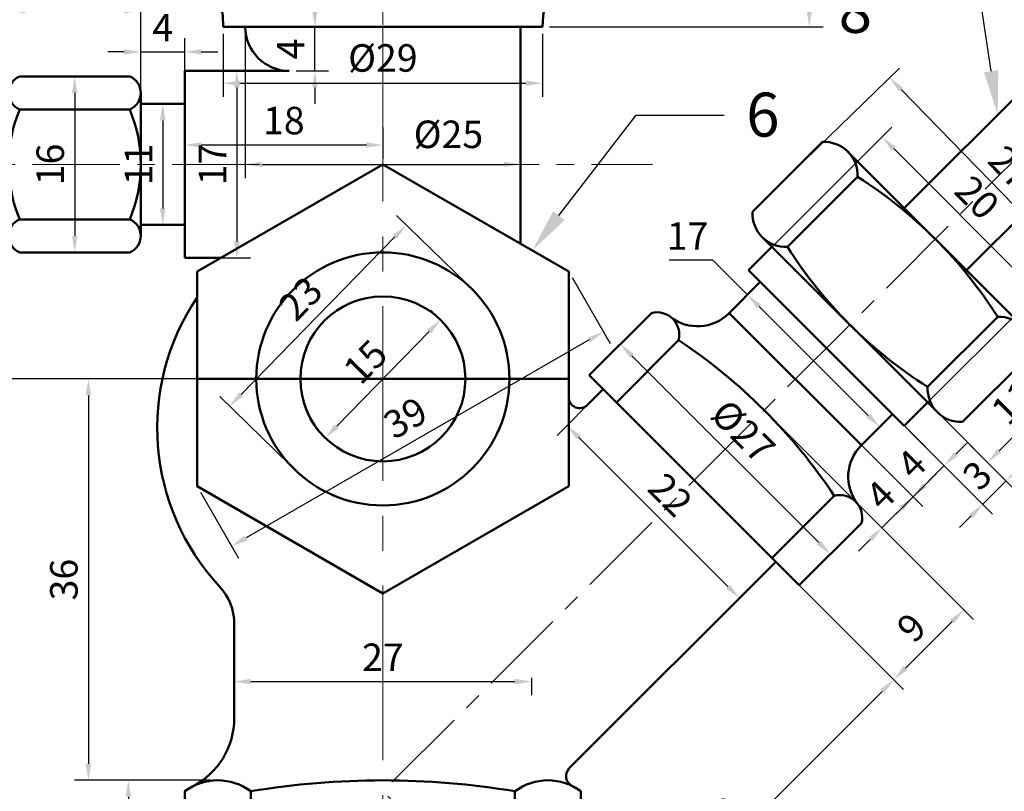
# Model space of a CAD drawing. Units: millimetres. Extents: x -414 to 17, y 81 to 417.
# Tile 3 of 7: x -341 to -252, y 143 to 214. Entities that reach past the tile are written whole.
import ezdxf
from ezdxf import colors
from ezdxf.entities.mleader import LeaderData, LeaderLine
from ezdxf.math import Vec2, Vec3

# ---------------------------------------------------------------- set-up
doc = ezdxf.new("R2010")
doc.units = ezdxf.units.MM
doc.header["$LTSCALE"] = 0.5
doc.linetypes.add('CENTER', pattern=[50.8, 31.75, -6.35, 6.35, -6.35])
for name, color, linetype, lineweight in [('M-CNTR', 1, 'CENTER', 18), ('M-DIMS', 2, 'Continuous', 25), ('M-OUTL', 7, 'Continuous', 50)]:
    doc.layers.add(name, color=color, linetype=linetype, lineweight=lineweight)
doc.styles.get("Standard").update_dxf_attribs({"font": 'arial.ttf'})
doc.dimstyles.new('ISO-25', dxfattribs={"dimtxt": 2.5, "dimasz": 1.5, "dimexe": 1.25, "dimexo": 0.625, "dimtad": 1, "dimtoh": 1, "dimdec": 0, "dimtxsty": 'Standard', "dimcen": 2.5, "dimadec": 0, "dimazin": 0, "dimtfac": 1, "dimtdec": 0, "dimtmove": 0, "dimatfit": 3, "dimfxl": 1, "dimarcsym": 0})

# ---------------------------------------------------------------- blocks, each defined once
blk = doc.blocks.new('*D20')
at = {"layer": 'Defpoints', "color": 0, "ltscale": 0.5, "transparency": 16777216}
for p in [(-281.414, 222.961), (-269.748, 222.961), (-293.993, 212.961)]:
    blk.add_point(p, dxfattribs=at)
at = {"layer": 'M-DIMS', "color": 0, "lineweight": -2, "ltscale": 0.5, "transparency": 16777216}
for p, q in [((-280.789, 222.961), (-268.498, 222.961)), ((-269.748, 214.461), (-269.748, 221.461)), ((-293.368, 212.961), (-268.498, 212.961))]:
    blk.add_line(p, q, dxfattribs=at)
at = {"layer": 'M-DIMS', "color": 0, "ltscale": 0.5, "transparency": 16777216}
for points in [[(-269.998, 221.461), (-269.498, 221.461), (-269.748, 222.961)], [(-269.998, 214.461), (-269.498, 214.461), (-269.748, 212.961)]]:
    blk.add_solid(points, dxfattribs=at)
at = {"layer": 'M-DIMS', "color": 0, "ltscale": 0.5, "transparency": 16777216, "insert": (-271.649, 217.961), "char_height": 2.5, "attachment_point": 5, "rotation": 90}
blk.add_mtext('10', dxfattribs=at)
blk = doc.blocks.new('*D23')
at = {"layer": 'Defpoints', "color": 0, "ltscale": 0.5, "transparency": 16777216}
for p in [(-322.993, 212.961), (-293.993, 212.961), (-293.993, 207.844)]:
    blk.add_point(p, dxfattribs=at)
at = {"layer": 'M-DIMS', "color": 0, "lineweight": -2, "ltscale": 0.5, "transparency": 16777216}
for p, q in [((-322.993, 212.336), (-322.993, 206.594)), ((-293.993, 212.336), (-293.993, 206.594)), ((-321.493, 207.844), (-295.493, 207.844))]:
    blk.add_line(p, q, dxfattribs=at)
at = {"layer": 'M-DIMS', "color": 0, "ltscale": 0.5, "transparency": 16777216}
for points in [[(-321.493, 208.094), (-321.493, 207.594), (-322.993, 207.844)], [(-295.493, 208.094), (-295.493, 207.594), (-293.993, 207.844)]]:
    blk.add_solid(points, dxfattribs=at)
at = {"layer": 'M-DIMS', "color": 0, "ltscale": 0.5, "transparency": 16777216, "insert": (-308.493, 209.815), "char_height": 2.5, "attachment_point": 5}
blk.add_mtext('%%C29', dxfattribs=at)
blk = doc.blocks.new('*D24')
at = {"layer": 'Defpoints', "color": 0, "ltscale": 0.5, "transparency": 16777216}
for p in [(-316.993, 212.961), (-314.671, 212.961), (-316.993, 208.961)]:
    blk.add_point(p, dxfattribs=at)
at = {"layer": 'M-DIMS', "color": 0, "lineweight": -2, "ltscale": 0.5, "transparency": 16777216}
for p, q in [((-314.671, 214.461), (-314.671, 215.961)), ((-316.368, 212.961), (-313.421, 212.961)), ((-314.671, 208.961), (-314.671, 212.961)), ((-316.368, 208.961), (-313.421, 208.961)), ((-314.671, 207.461), (-314.671, 205.961))]:
    blk.add_line(p, q, dxfattribs=at)
at = {"layer": 'M-DIMS', "color": 0, "ltscale": 0.5, "transparency": 16777216}
for points in [[(-314.921, 214.461), (-314.421, 214.461), (-314.671, 212.961)], [(-314.921, 207.461), (-314.421, 207.461), (-314.671, 208.961)]]:
    blk.add_solid(points, dxfattribs=at)
at = {"layer": 'M-DIMS', "color": 0, "ltscale": 0.5, "transparency": 16777216, "insert": (-316.546, 210.961), "char_height": 2.5, "attachment_point": 5, "rotation": 90}
blk.add_mtext('4', dxfattribs=at)
blk = doc.blocks.new('*D25')
at = {"layer": 'Defpoints', "color": 0, "ltscale": 0.5, "transparency": 16777216}
for p in [(-326.493, 204.436), (-308.493, 204.436), (-326.493, 202.223)]:
    blk.add_point(p, dxfattribs=at)
at = {"layer": 'M-DIMS', "color": 0, "lineweight": -2, "ltscale": 0.5, "transparency": 16777216}
for p, q in [((-326.493, 203.811), (-326.493, 200.973)), ((-308.493, 203.811), (-308.493, 200.973)), ((-309.993, 202.223), (-324.993, 202.223))]:
    blk.add_line(p, q, dxfattribs=at)
at = {"layer": 'M-DIMS', "color": 0, "ltscale": 0.5, "transparency": 16777216}
for points in [[(-324.993, 202.473), (-324.993, 201.973), (-326.493, 202.223)], [(-309.993, 202.473), (-309.993, 201.973), (-308.493, 202.223)]]:
    blk.add_solid(points, dxfattribs=at)
at = {"layer": 'M-DIMS', "color": 0, "ltscale": 0.5, "transparency": 16777216, "insert": (-317.493, 204.125), "char_height": 2.5, "attachment_point": 5}
blk.add_mtext('18', dxfattribs=at)
blk = doc.blocks.new('*D26')
at = {"layer": 'Defpoints', "color": 0, "ltscale": 0.5, "transparency": 16777216}
for p in [(-320.993, 212.961), (-295.993, 203.103), (-295.993, 200.461)]:
    blk.add_point(p, dxfattribs=at)
at = {"layer": 'M-DIMS', "color": 0, "lineweight": -2, "ltscale": 0.5, "transparency": 16777216}
for p, q in [((-320.993, 212.336), (-320.993, 199.211)), ((-295.993, 202.478), (-295.993, 199.211)), ((-319.493, 200.461), (-297.493, 200.461))]:
    blk.add_line(p, q, dxfattribs=at)
at = {"layer": 'M-DIMS', "color": 0, "ltscale": 0.5, "transparency": 16777216}
for points in [[(-319.493, 200.711), (-319.493, 200.211), (-320.993, 200.461)], [(-297.493, 200.711), (-297.493, 200.211), (-295.993, 200.461)]]:
    blk.add_solid(points, dxfattribs=at)
at = {"layer": 'M-DIMS', "color": 0, "ltscale": 0.5, "transparency": 16777216, "insert": (-302.537, 202.873), "char_height": 2.5, "attachment_point": 5}
blk.add_mtext('%%C25', dxfattribs=at)
blk = doc.blocks.new('*D27')
at = {"layer": 'Defpoints', "color": 0, "ltscale": 0.5, "transparency": 16777216}
for p in [(-325.219, 208.961), (-325.219, 191.961), (-321.764, 191.961)]:
    blk.add_point(p, dxfattribs=at)
at = {"layer": 'M-DIMS', "color": 0, "lineweight": -2, "ltscale": 0.5, "transparency": 16777216}
for p, q in [((-324.594, 208.961), (-320.514, 208.961)), ((-321.764, 207.461), (-321.764, 193.461)), ((-324.594, 191.961), (-320.514, 191.961))]:
    blk.add_line(p, q, dxfattribs=at)
at = {"layer": 'M-DIMS', "color": 0, "ltscale": 0.5, "transparency": 16777216}
for points in [[(-322.014, 207.461), (-321.514, 207.461), (-321.764, 208.961)], [(-322.014, 193.461), (-321.514, 193.461), (-321.764, 191.961)]]:
    blk.add_solid(points, dxfattribs=at)
at = {"layer": 'M-DIMS', "color": 0, "ltscale": 0.5, "transparency": 16777216, "insert": (-323.644, 200.461), "char_height": 2.5, "attachment_point": 5, "rotation": 90}
blk.add_mtext('17', dxfattribs=at)
blk = doc.blocks.new('*D28')
at = {"layer": 'Defpoints', "color": 0, "ltscale": 0.5, "transparency": 16777216}
for p in [(-328.493, 205.961), (-328.493, 194.961), (-328.493, 194.961)]:
    blk.add_point(p, dxfattribs=at)
at = {"layer": 'M-DIMS', "color": 0, "lineweight": -2, "ltscale": 0.5, "transparency": 16777216}
for p, q in [((-329.118, 205.961), (-329.743, 205.961)), ((-328.493, 204.461), (-328.493, 196.461)), ((-329.118, 194.961), (-329.743, 194.961))]:
    blk.add_line(p, q, dxfattribs=at)
at = {"layer": 'M-DIMS', "color": 0, "ltscale": 0.5, "transparency": 16777216}
for points in [[(-328.743, 204.461), (-328.243, 204.461), (-328.493, 205.961)], [(-328.743, 196.461), (-328.243, 196.461), (-328.493, 194.961)]]:
    blk.add_solid(points, dxfattribs=at)
at = {"layer": 'M-DIMS', "color": 0, "ltscale": 0.5, "transparency": 16777216, "insert": (-330.373, 200.461), "char_height": 2.5, "attachment_point": 5, "rotation": 90}
blk.add_mtext('11', dxfattribs=at)
blk = doc.blocks.new('*D29')
at = {"layer": 'Defpoints', "color": 0, "ltscale": 0.5, "transparency": 16777216}
for p in [(-326.493, 210.694), (-330.493, 205.961), (-326.493, 205.961)]:
    blk.add_point(p, dxfattribs=at)
at = {"layer": 'M-DIMS', "color": 0, "lineweight": -2, "ltscale": 0.5, "transparency": 16777216}
for p, q in [((-330.493, 206.586), (-330.493, 211.944)), ((-326.493, 206.586), (-326.493, 211.944)), ((-331.993, 210.694), (-333.493, 210.694)), ((-330.493, 210.694), (-326.493, 210.694)), ((-324.993, 210.694), (-323.493, 210.694))]:
    blk.add_line(p, q, dxfattribs=at)
at = {"layer": 'M-DIMS', "color": 0, "ltscale": 0.5, "transparency": 16777216}
for points in [[(-331.993, 210.944), (-331.993, 210.444), (-330.493, 210.694)], [(-324.993, 210.944), (-324.993, 210.444), (-326.493, 210.694)]]:
    blk.add_solid(points, dxfattribs=at)
at = {"layer": 'M-DIMS', "color": 0, "ltscale": 0.5, "transparency": 16777216, "insert": (-328.493, 212.569), "char_height": 2.5, "attachment_point": 5}
blk.add_mtext('4', dxfattribs=at)
blk = doc.blocks.new('*D30')
at = {"layer": 'Defpoints', "color": 0, "ltscale": 0.5, "transparency": 16777216}
for p in [(-330.493, 214.444), (-330.493, 209.265), (-342.493, 205.101)]:
    blk.add_point(p, dxfattribs=at)
at = {"layer": 'M-DIMS', "color": 0, "lineweight": -2, "ltscale": 0.5, "transparency": 16777216}
for p, q in [((-342.493, 205.726), (-342.493, 215.694)), ((-330.493, 209.89), (-330.493, 215.694)), ((-340.993, 214.444), (-331.993, 214.444))]:
    blk.add_line(p, q, dxfattribs=at)
at = {"layer": 'M-DIMS', "color": 0, "ltscale": 0.5, "transparency": 16777216}
for points in [[(-340.993, 214.694), (-340.993, 214.194), (-342.493, 214.444)], [(-331.993, 214.694), (-331.993, 214.194), (-330.493, 214.444)]]:
    blk.add_solid(points, dxfattribs=at)
at = {"layer": 'M-DIMS', "color": 0, "ltscale": 0.5, "transparency": 16777216, "insert": (-336.493, 216.324), "char_height": 2.5, "attachment_point": 5}
blk.add_mtext('12', dxfattribs=at)
blk = doc.blocks.new('*D31')
at = {"layer": 'Defpoints', "color": 0, "ltscale": 0.5, "transparency": 16777216}
for p in [(-336.493, 208.461), (-336.493, 192.461), (-336.493, 192.461)]:
    blk.add_point(p, dxfattribs=at)
at = {"layer": 'M-DIMS', "color": 0, "lineweight": -2, "ltscale": 0.5, "transparency": 16777216}
for p, q in [((-337.118, 208.461), (-337.743, 208.461)), ((-336.493, 206.961), (-336.493, 193.961)), ((-337.118, 192.461), (-337.743, 192.461))]:
    blk.add_line(p, q, dxfattribs=at)
at = {"layer": 'M-DIMS', "color": 0, "ltscale": 0.5, "transparency": 16777216}
for points in [[(-336.743, 206.961), (-336.243, 206.961), (-336.493, 208.461)], [(-336.743, 193.961), (-336.243, 193.961), (-336.493, 192.461)]]:
    blk.add_solid(points, dxfattribs=at)
at = {"layer": 'M-DIMS', "color": 0, "ltscale": 0.5, "transparency": 16777216, "insert": (-338.394, 200.461), "char_height": 2.5, "attachment_point": 5, "rotation": 90}
blk.add_mtext('16', dxfattribs=at)
blk = doc.blocks.new('*D37')
at = {"layer": 'Defpoints', "color": 0, "ltscale": 0.5, "transparency": 16777216}
for p in [(-338.493, 222.961), (-374.146, 180.961), (-308.493, 180.961)]:
    blk.add_point(p, dxfattribs=at)
at = {"layer": 'M-DIMS', "color": 0, "lineweight": -2, "ltscale": 0.5, "transparency": 16777216}
for p, q in [((-339.118, 222.961), (-375.396, 222.961)), ((-374.146, 221.461), (-374.146, 182.461)), ((-309.118, 180.961), (-375.396, 180.961))]:
    blk.add_line(p, q, dxfattribs=at)
at = {"layer": 'M-DIMS', "color": 0, "ltscale": 0.5, "transparency": 16777216}
for points in [[(-374.396, 221.461), (-373.896, 221.461), (-374.146, 222.961)], [(-374.396, 182.461), (-373.896, 182.461), (-374.146, 180.961)]]:
    blk.add_solid(points, dxfattribs=at)
at = {"layer": 'M-DIMS', "color": 0, "ltscale": 0.5, "transparency": 16777216, "insert": (-376.027, 201.961), "char_height": 2.5, "attachment_point": 5, "rotation": 90}
blk.add_mtext('42', dxfattribs=at)
blk = doc.blocks.new('*D41')
at = {"layer": 'Defpoints', "color": 0, "ltscale": 0.5, "transparency": 16777216}
for p in [(-383.576, 200.461), (-351.797, 200.461), (-308.493, 115.461)]:
    blk.add_point(p, dxfattribs=at)
at = {"layer": 'M-DIMS', "color": 0, "lineweight": -2, "ltscale": 0.5, "transparency": 16777216}
for p, q in [((-352.422, 200.461), (-384.826, 200.461)), ((-383.576, 116.961), (-383.576, 198.961)), ((-309.118, 115.461), (-384.826, 115.461))]:
    blk.add_line(p, q, dxfattribs=at)
at = {"layer": 'M-DIMS', "color": 0, "ltscale": 0.5, "transparency": 16777216}
for points in [[(-383.826, 198.961), (-383.326, 198.961), (-383.576, 200.461)], [(-383.826, 116.961), (-383.326, 116.961), (-383.576, 115.461)]]:
    blk.add_solid(points, dxfattribs=at)
at = {"layer": 'M-DIMS', "color": 0, "ltscale": 0.5, "transparency": 16777216, "insert": (-385.477, 157.961), "char_height": 2.5, "attachment_point": 5, "rotation": 90}
blk.add_mtext('85', dxfattribs=at)
blk = doc.blocks.new('*D44')
at = {"layer": 'Defpoints', "color": 0, "ltscale": 0.5, "transparency": 16777216}
for p in [(-334.948, 180.961), (-335.25, 144.461), (-323.493, 144.461)]:
    blk.add_point(p, dxfattribs=at)
at = {"layer": 'M-DIMS', "color": 0, "lineweight": -2, "ltscale": 0.5, "transparency": 16777216}
for p, q in [((-335.573, 180.961), (-336.5, 180.961)), ((-335.25, 179.461), (-335.25, 145.961)), ((-324.118, 144.461), (-336.5, 144.461))]:
    blk.add_line(p, q, dxfattribs=at)
at = {"layer": 'M-DIMS', "color": 0, "ltscale": 0.5, "transparency": 16777216}
for points in [[(-335.5, 179.461), (-335, 179.461), (-335.25, 180.961)], [(-335.5, 145.961), (-335, 145.961), (-335.25, 144.461)]]:
    blk.add_solid(points, dxfattribs=at)
at = {"layer": 'M-DIMS', "color": 0, "ltscale": 0.5, "transparency": 16777216, "insert": (-337.153, 162.711), "char_height": 2.5, "attachment_point": 5, "rotation": 90}
blk.add_mtext('36', dxfattribs=at)
blk = doc.blocks.new('*D47')
at = {"layer": 'Defpoints', "color": 0, "ltscale": 0.5, "transparency": 16777216}
for p in [(-323.493, 144.461), (-331.619, 133.461), (-323.493, 133.461)]:
    blk.add_point(p, dxfattribs=at)
at = {"layer": 'M-DIMS', "color": 0, "lineweight": -2, "ltscale": 0.5, "transparency": 16777216}
for p, q in [((-324.118, 144.461), (-332.869, 144.461)), ((-331.619, 142.961), (-331.619, 134.961)), ((-324.118, 133.461), (-332.869, 133.461))]:
    blk.add_line(p, q, dxfattribs=at)
at = {"layer": 'M-DIMS', "color": 0, "ltscale": 0.5, "transparency": 16777216}
for points in [[(-331.869, 142.961), (-331.369, 142.961), (-331.619, 144.461)], [(-331.869, 134.961), (-331.369, 134.961), (-331.619, 133.461)]]:
    blk.add_solid(points, dxfattribs=at)
at = {"layer": 'M-DIMS', "color": 0, "ltscale": 0.5, "transparency": 16777216, "insert": (-333.499, 138.961), "char_height": 2.5, "attachment_point": 5, "rotation": 90}
blk.add_mtext('11', dxfattribs=at)
blk = doc.blocks.new('*D49')
at = {"layer": 'Defpoints', "color": 0, "ltscale": 0.5, "transparency": 16777216}
for p in [(-321.993, 154.405), (-294.993, 154.405), (-294.993, 153.443)]:
    blk.add_point(p, dxfattribs=at)
at = {"layer": 'M-DIMS', "color": 0, "lineweight": -2, "ltscale": 0.5, "transparency": 16777216}
for p, q in [((-321.993, 153.78), (-321.993, 152.193)), ((-320.493, 153.443), (-296.493, 153.443)), ((-294.993, 153.78), (-294.993, 152.193))]:
    blk.add_line(p, q, dxfattribs=at)
at = {"layer": 'M-DIMS', "color": 0, "ltscale": 0.5, "transparency": 16777216}
for points in [[(-320.493, 153.693), (-320.493, 153.193), (-321.993, 153.443)], [(-296.493, 153.693), (-296.493, 153.193), (-294.993, 153.443)]]:
    blk.add_solid(points, dxfattribs=at)
at = {"layer": 'M-DIMS', "color": 0, "ltscale": 0.5, "transparency": 16777216, "insert": (-308.493, 155.323), "char_height": 2.5, "attachment_point": 5}
blk.add_mtext('27', dxfattribs=at)
blk = doc.blocks.new('*D59')
at = {"layer": 'Defpoints', "color": 0, "ltscale": 0.5, "transparency": 16777216}
for p in [(-250.176, 185.541), (-257.948, 177.769), (-253.55, 173.371)]:
    blk.add_point(p, dxfattribs=at)
at = {"layer": 'M-DIMS', "color": 0, "lineweight": -2, "ltscale": 0.5, "transparency": 16777216}
for p, q in [((-249.734, 185.099), (-244.894, 180.259)), ((-246.839, 180.083), (-252.489, 174.432)), ((-257.506, 177.328), (-252.666, 172.487))]:
    blk.add_line(p, q, dxfattribs=at)
at = {"layer": 'M-DIMS', "color": 0, "ltscale": 0.5, "transparency": 16777216}
for points in [[(-247.015, 180.259), (-246.662, 179.906), (-245.778, 181.143)], [(-252.666, 174.609), (-252.313, 174.255), (-253.55, 173.371)]]:
    blk.add_solid(points, dxfattribs=at)
at = {"layer": 'M-DIMS', "color": 0, "ltscale": 0.5, "transparency": 16777216, "insert": (-250.993, 178.587), "char_height": 2.5, "attachment_point": 5, "rotation": 45}
blk.add_mtext('11', dxfattribs=at)
blk = doc.blocks.new('*D60')
at = {"layer": 'Defpoints', "color": 0, "ltscale": 0.5, "transparency": 16777216}
for p in [(-271.723, 199.323), (-243.626, 188.985), (-252.893, 179.969)]:
    blk.add_point(p, dxfattribs=at)
at = {"layer": 'M-DIMS', "color": 0, "lineweight": -2, "ltscale": 0.5, "transparency": 16777216}
for p, q in [((-271.275, 199.759), (-261.56, 209.211)), ((-261.41, 207.264), (-244.672, 190.06)), ((-252.445, 180.405), (-242.73, 189.857))]:
    blk.add_line(p, q, dxfattribs=at)
at = {"layer": 'M-DIMS', "color": 0, "ltscale": 0.5, "transparency": 16777216}
for points in [[(-261.231, 207.438), (-261.589, 207.09), (-262.456, 208.339)], [(-244.493, 190.235), (-244.851, 189.886), (-243.626, 188.985)]]:
    blk.add_solid(points, dxfattribs=at)
at = {"layer": 'M-DIMS', "color": 0, "ltscale": 0.5, "transparency": 16777216, "insert": (-251.693, 199.973), "char_height": 2.5, "attachment_point": 5, "rotation": 314.21384}
blk.add_mtext('27', dxfattribs=at)
blk = doc.blocks.new('*D61')
at = {"layer": 'Defpoints', "color": 0, "ltscale": 0.5, "transparency": 16777216}
for p in [(-274.198, 191.898), (-248.999, 188.813), (-260.056, 177.756)]:
    blk.add_point(p, dxfattribs=at)
at = {"layer": 'M-DIMS', "color": 0, "lineweight": -2, "ltscale": 0.5, "transparency": 16777216}
for p, q in [((-273.756, 192.34), (-262.257, 203.839)), ((-262.08, 201.894), (-250.06, 189.873)), ((-259.614, 178.198), (-248.115, 189.697))]:
    blk.add_line(p, q, dxfattribs=at)
at = {"layer": 'M-DIMS', "color": 0, "ltscale": 0.5, "transparency": 16777216}
for points in [[(-261.904, 202.071), (-262.257, 201.717), (-263.141, 202.955)], [(-249.883, 190.05), (-250.236, 189.697), (-248.999, 188.813)]]:
    blk.add_solid(points, dxfattribs=at)
at = {"layer": 'M-DIMS', "color": 0, "ltscale": 0.5, "transparency": 16777216, "insert": (-254.726, 197.228), "char_height": 2.5, "attachment_point": 5, "rotation": 315}
blk.add_mtext('20', dxfattribs=at)
blk = doc.blocks.new('*D62')
at = {"layer": 'Defpoints', "color": 0, "ltscale": 0.5, "transparency": 16777216}
for p in [(-275.629, 188.346), (-263.608, 176.325), (-263.348, 176.585)]:
    blk.add_point(p, dxfattribs=at)
at = {"layer": 'M-DIMS', "color": 0, "lineweight": -2, "ltscale": 0.5, "transparency": 16777216}
for p, q in [((-278.508, 191.746), (-282.479, 191.746)), ((-275.369, 188.606), (-278.508, 191.746)), ((-275.187, 188.788), (-274.485, 189.49)), ((-264.409, 177.646), (-274.308, 187.545)), ((-263.166, 176.767), (-262.464, 177.469))]:
    blk.add_line(p, q, dxfattribs=at)
at = {"layer": 'M-DIMS', "color": 0, "ltscale": 0.5, "transparency": 16777216}
for points in [[(-274.131, 187.722), (-274.485, 187.369), (-275.369, 188.606)], [(-264.232, 177.823), (-264.585, 177.469), (-263.348, 176.585)]]:
    blk.add_solid(points, dxfattribs=at)
at = {"layer": 'M-DIMS', "color": 0, "ltscale": 0.5, "transparency": 16777216, "insert": (-280.806, 193.626), "char_height": 2.5, "attachment_point": 5}
blk.add_mtext('17', dxfattribs=at)
blk = doc.blocks.new('*D63')
at = {"layer": 'Defpoints', "color": 0, "ltscale": 0.5, "transparency": 16777216}
for p in [(-286.926, 184.12), (-267.834, 165.028), (-267.834, 165.028)]:
    blk.add_point(p, dxfattribs=at)
at = {"layer": 'M-DIMS', "color": 0, "lineweight": -2, "ltscale": 0.5, "transparency": 16777216}
for p, q in [((-286.484, 184.562), (-286.042, 185.004)), ((-285.865, 183.059), (-268.895, 166.089)), ((-267.392, 165.47), (-266.95, 165.912))]:
    blk.add_line(p, q, dxfattribs=at)
at = {"layer": 'M-DIMS', "color": 0, "ltscale": 0.5, "transparency": 16777216}
for points in [[(-285.688, 183.236), (-286.042, 182.882), (-286.926, 184.12)], [(-268.718, 166.265), (-269.071, 165.912), (-267.834, 165.028)]]:
    blk.add_solid(points, dxfattribs=at)
at = {"layer": 'M-DIMS', "color": 0, "ltscale": 0.5, "transparency": 16777216, "insert": (-275.986, 175.968), "char_height": 2.5, "attachment_point": 5, "rotation": 315}
blk.add_mtext('%%C27', dxfattribs=at)
blk = doc.blocks.new('*D64')
at = {"layer": 'Defpoints', "color": 0, "ltscale": 0.5, "transparency": 16777216}
for p in [(-265.368, 169.611), (-271.721, 163.258), (-262.07, 153.607)]:
    blk.add_point(p, dxfattribs=at)
at = {"layer": 'M-DIMS', "color": 0, "lineweight": -2, "ltscale": 0.5, "transparency": 16777216}
for p, q in [((-264.927, 169.169), (-254.833, 159.076)), ((-271.279, 162.816), (-261.186, 152.723)), ((-256.778, 158.899), (-261.009, 154.668))]:
    blk.add_line(p, q, dxfattribs=at)
at = {"layer": 'M-DIMS', "color": 0, "ltscale": 0.5, "transparency": 16777216}
for points in [[(-256.954, 159.076), (-256.601, 158.722), (-255.717, 159.96)], [(-261.186, 154.844), (-260.832, 154.491), (-262.07, 153.607)]]:
    blk.add_solid(points, dxfattribs=at)
at = {"layer": 'M-DIMS', "color": 0, "ltscale": 0.5, "transparency": 16777216, "insert": (-260.238, 158.128), "char_height": 2.5, "attachment_point": 5, "rotation": 45}
blk.add_mtext('9', dxfattribs=at)
blk = doc.blocks.new('*D65')
at = {"layer": 'Defpoints', "color": 0, "ltscale": 0.5, "transparency": 16777216}
for p in [(-271.016, 180.938), (-273.844, 178.109), (-260.323, 170.245)]:
    blk.add_point(p, dxfattribs=at)
at = {"layer": 'M-DIMS', "color": 0, "lineweight": -2, "ltscale": 0.5, "transparency": 16777216}
for p, q in [((-270.574, 180.496), (-259.439, 169.361)), ((-273.402, 177.668), (-262.267, 166.533)), ((-259.262, 171.305), (-258.202, 172.366)), ((-263.151, 167.416), (-260.323, 170.245)), ((-264.212, 166.356), (-265.273, 165.295))]:
    blk.add_line(p, q, dxfattribs=at)
at = {"layer": 'M-DIMS', "color": 0, "ltscale": 0.5, "transparency": 16777216}
for points in [[(-259.439, 171.482), (-259.085, 171.129), (-260.323, 170.245)], [(-264.389, 166.533), (-264.035, 166.179), (-263.151, 167.416)]]:
    blk.add_solid(points, dxfattribs=at)
at = {"layer": 'M-DIMS', "color": 0, "ltscale": 0.5, "transparency": 16777216, "insert": (-263.063, 170.156), "char_height": 2.5, "attachment_point": 5, "rotation": 45}
blk.add_mtext('4', dxfattribs=at)
blk = doc.blocks.new('*D66')
at = {"layer": 'Defpoints', "color": 0, "ltscale": 0.5, "transparency": 16777216}
for p in [(-262.177, 177.756), (-265.007, 174.928), (-257.495, 173.071)]:
    blk.add_point(p, dxfattribs=at)
at = {"layer": 'M-DIMS', "color": 0, "lineweight": -2, "ltscale": 0.5, "transparency": 16777216}
for p, q in [((-261.735, 177.314), (-256.612, 172.187)), ((-264.565, 174.486), (-259.441, 169.359)), ((-256.434, 174.131), (-255.373, 175.191)), ((-260.324, 170.243), (-257.495, 173.071)), ((-261.385, 169.183), (-262.446, 168.123))]:
    blk.add_line(p, q, dxfattribs=at)
at = {"layer": 'M-DIMS', "color": 0, "ltscale": 0.5, "transparency": 16777216}
for points in [[(-256.611, 174.308), (-256.257, 173.954), (-257.495, 173.071)], [(-261.562, 169.36), (-261.209, 169.006), (-260.324, 170.243)]]:
    blk.add_solid(points, dxfattribs=at)
at = {"layer": 'M-DIMS', "color": 0, "ltscale": 0.5, "transparency": 16777216, "insert": (-260.235, 172.983), "char_height": 2.5, "attachment_point": 5, "rotation": 44.98084}
blk.add_mtext('4', dxfattribs=at)
blk = doc.blocks.new('*D67')
at = {"layer": 'Defpoints', "color": 0, "ltscale": 0.5, "transparency": 16777216}
for p in [(-258.995, 178.817), (-261.117, 176.695), (-251.858, 171.68)]:
    blk.add_point(p, dxfattribs=at)
at = {"layer": 'M-DIMS', "color": 0, "lineweight": -2, "ltscale": 0.5, "transparency": 16777216}
for p, q in [((-258.553, 178.375), (-250.974, 170.796)), ((-260.675, 176.253), (-253.096, 168.674)), ((-250.798, 172.74), (-249.737, 173.801)), ((-253.98, 169.558), (-251.858, 171.68)), ((-255.04, 168.498), (-256.101, 167.437))]:
    blk.add_line(p, q, dxfattribs=at)
at = {"layer": 'M-DIMS', "color": 0, "ltscale": 0.5, "transparency": 16777216}
for points in [[(-250.974, 172.917), (-250.621, 172.563), (-251.858, 171.68)], [(-255.217, 168.674), (-254.863, 168.321), (-253.98, 169.558)]]:
    blk.add_solid(points, dxfattribs=at)
at = {"layer": 'M-DIMS', "color": 0, "ltscale": 0.5, "transparency": 16777216, "insert": (-254.264, 171.964), "char_height": 2.5, "attachment_point": 5, "rotation": 45}
blk.add_mtext('3', dxfattribs=at)
blk = doc.blocks.new('*D68')
at = {"layer": 'Defpoints', "color": 0, "ltscale": 0.5, "transparency": 16777216}
for p in [(-288.475, 180.012), (-272.784, 164.321), (-276.084, 161.02)]:
    blk.add_point(p, dxfattribs=at)
at = {"layer": 'M-DIMS', "color": 0, "lineweight": -2, "ltscale": 0.5, "transparency": 16777216}
for p, q in [((-288.917, 179.57), (-292.659, 175.827)), ((-290.714, 175.651), (-277.145, 162.081)), ((-273.226, 163.879), (-276.968, 160.136))]:
    blk.add_line(p, q, dxfattribs=at)
at = {"layer": 'M-DIMS', "color": 0, "ltscale": 0.5, "transparency": 16777216}
for points in [[(-290.538, 175.827), (-290.891, 175.474), (-291.775, 176.711)], [(-276.968, 162.258), (-277.322, 161.904), (-276.084, 161.02)]]:
    blk.add_solid(points, dxfattribs=at)
at = {"layer": 'M-DIMS', "color": 0, "ltscale": 0.5, "transparency": 16777216, "insert": (-282.6, 170.195), "char_height": 2.5, "attachment_point": 5, "rotation": 315}
blk.add_mtext('22', dxfattribs=at)
blk = doc.blocks.new('*D69')
at = {"layer": 'Defpoints', "color": 0, "ltscale": 0.5, "transparency": 16777216}
for p in [(-280.208, 171.746), (-262.07, 153.607), (-308.493, 143.461)]:
    blk.add_point(p, dxfattribs=at)
at = {"layer": 'M-DIMS', "color": 0, "lineweight": -2, "ltscale": 0.5, "transparency": 16777216}
for p, q in [((-279.766, 171.304), (-261.186, 152.723)), ((-289.293, 126.383), (-263.13, 152.546)), ((-308.051, 143.019), (-289.47, 124.439))]:
    blk.add_line(p, q, dxfattribs=at)
at = {"layer": 'M-DIMS', "color": 0, "ltscale": 0.5, "transparency": 16777216}
for points in [[(-263.307, 152.723), (-262.954, 152.369), (-262.07, 153.607)], [(-289.47, 126.56), (-289.117, 126.207), (-290.354, 125.323)]]:
    blk.add_solid(points, dxfattribs=at)
at = {"layer": 'M-DIMS', "color": 0, "ltscale": 0.5, "transparency": 16777216, "insert": (-277.556, 140.809), "char_height": 2.5, "attachment_point": 5, "rotation": 45}
blk.add_mtext('40', dxfattribs=at)
blk = doc.blocks.new('*D70')
at = {"layer": 'Defpoints', "color": 0, "ltscale": 0.5, "transparency": 16777216}
for p in [(-222.226, 229.728), (-308.493, 143.461), (-278.374, 113.343)]:
    blk.add_point(p, dxfattribs=at)
at = {"layer": 'M-DIMS', "color": 0, "lineweight": -2, "ltscale": 0.5, "transparency": 16777216}
for p, q in [((-221.784, 229.286), (-191.223, 198.726)), ((-193.168, 198.549), (-277.314, 114.404)), ((-308.051, 143.019), (-277.49, 112.459))]:
    blk.add_line(p, q, dxfattribs=at)
at = {"layer": 'M-DIMS', "color": 0, "ltscale": 0.5, "transparency": 16777216}
for points in [[(-193.345, 198.726), (-192.991, 198.373), (-192.107, 199.61)], [(-277.49, 114.58), (-277.137, 114.227), (-278.374, 113.343)]]:
    blk.add_solid(points, dxfattribs=at)
at = {"layer": 'M-DIMS', "color": 0, "ltscale": 0.5, "transparency": 16777216, "insert": (-236.57, 157.806), "char_height": 2.5, "attachment_point": 5, "rotation": 45}
blk.add_mtext('122', dxfattribs=at)
blk = doc.blocks.new('*D78')
at = {"layer": 'Defpoints', "color": 0, "ltscale": 0.5, "transparency": 16777216}
for p in [(-308.493, 365.429), (-250.629, 243.684), (-212.22, 239.734), (-308.493, 230.961), (-308.493, 143.461)]:
    blk.add_point(p, dxfattribs=at)
at = {"layer": 'M-DIMS', "color": 0, "lineweight": -2, "ltscale": 0.5, "transparency": 16777216}
blk.add_arc((-308.493, 143.461), 115.727, 45.74265, 89.25735, dxfattribs=at)
at = {"layer": 'M-DIMS', "color": 0, "ltscale": 0.5, "transparency": 16777216}
for points in [[(-306.994, 258.928), (-306.991, 259.428), (-308.493, 259.188)], [(-227.553, 226.524), (-227.905, 226.168), (-226.662, 225.292)]]:
    blk.add_solid(points, dxfattribs=at)
at = {"layer": 'M-DIMS', "color": 0, "ltscale": 0.5, "transparency": 16777216, "insert": (-263.48, 252.131), "char_height": 2.5, "attachment_point": 5, "rotation": 337.5}
blk.add_mtext('45°', dxfattribs=at)
blk = doc.blocks.new('*D79')
at = {"layer": 'Defpoints', "color": 0, "ltscale": 0.5, "transparency": 16777216}
for p in [(-303.255, 186.329), (-313.731, 175.594), (-313.731, 175.594)]:
    blk.add_point(p, dxfattribs=at)
at = {"layer": 'M-DIMS', "color": 0, "lineweight": -2, "ltscale": 0.5, "transparency": 16777216}
for p, q in [((-303.702, 186.765), (-304.149, 187.202)), ((-304.302, 185.255), (-312.683, 176.667)), ((-314.178, 176.03), (-314.625, 176.467))]:
    blk.add_line(p, q, dxfattribs=at)
at = {"layer": 'M-DIMS', "color": 0, "ltscale": 0.5, "transparency": 16777216}
for points in [[(-304.481, 185.43), (-304.123, 185.081), (-303.255, 186.329)], [(-312.862, 176.842), (-312.504, 176.492), (-313.731, 175.594)]]:
    blk.add_solid(points, dxfattribs=at)
at = {"layer": 'M-DIMS', "color": 0, "ltscale": 0.5, "transparency": 16777216, "insert": (-309.854, 182.289), "char_height": 2.5, "attachment_point": 5, "rotation": 45.70011}
blk.add_mtext('15', dxfattribs=at)
blk = doc.blocks.new('*D80')
at = {"layer": 'Defpoints', "color": 0, "ltscale": 0.5, "transparency": 16777216}
for p in [(-300.461, 189.192), (-322.415, 178.479), (-316.524, 172.731)]:
    blk.add_point(p, dxfattribs=at)
at = {"layer": 'M-DIMS', "color": 0, "lineweight": -2, "ltscale": 0.5, "transparency": 16777216}
for p, q in [((-300.908, 189.628), (-307.246, 195.813)), ((-307.399, 193.866), (-321.367, 179.553)), ((-316.972, 173.167), (-323.31, 179.352))]:
    blk.add_line(p, q, dxfattribs=at)
at = {"layer": 'M-DIMS', "color": 0, "ltscale": 0.5, "transparency": 16777216}
for points in [[(-307.578, 194.041), (-307.22, 193.692), (-306.351, 194.94)], [(-321.546, 179.727), (-321.188, 179.378), (-322.415, 178.479)]]:
    blk.add_solid(points, dxfattribs=at)
at = {"layer": 'M-DIMS', "color": 0, "ltscale": 0.5, "transparency": 16777216, "insert": (-315.745, 188.038), "char_height": 2.5, "attachment_point": 5, "rotation": 45.70011}
blk.add_mtext('23', dxfattribs=at)
blk = doc.blocks.new('*D81')
at = {"layer": 'Defpoints', "color": 0, "ltscale": 0.5, "transparency": 16777216}
for p in [(-291.605, 190.711), (-325.38, 171.211), (-322.227, 165.75)]:
    blk.add_point(p, dxfattribs=at)
at = {"layer": 'M-DIMS', "color": 0, "lineweight": -2, "ltscale": 0.5, "transparency": 16777216}
for p, q in [((-291.293, 190.17), (-287.827, 184.167)), ((-289.751, 184.5), (-320.928, 166.5)), ((-325.068, 170.67), (-321.602, 164.667))]:
    blk.add_line(p, q, dxfattribs=at)
at = {"layer": 'M-DIMS', "color": 0, "ltscale": 0.5, "transparency": 16777216}
for points in [[(-289.876, 184.716), (-289.626, 184.283), (-288.452, 185.25)], [(-321.053, 166.716), (-320.803, 166.283), (-322.227, 165.75)]]:
    blk.add_solid(points, dxfattribs=at)
at = {"layer": 'M-DIMS', "color": 0, "ltscale": 0.5, "transparency": 16777216, "insert": (-306.291, 177.147), "char_height": 2.5, "attachment_point": 5, "rotation": 30}
blk.add_mtext('39', dxfattribs=at)

msp = doc.modelspace()

# ---------------------------------------------------------------- linework, layer by layer
at = {"layer": 'M-CNTR', "ltscale": 0.5}
for p, q in [((-212.22, 239.734), (-308.493, 143.461)), ((-308.493, 200.461), (-308.493, 230.961)), ((-365.728, 200.461), (-283.993, 200.461))]:
    msp.add_line(p, q, dxfattribs=at)
at = {"layer": 'M-CNTR'}
msp.add_line((-308.493, 212.961), (-308.493, 102.529), dxfattribs=at)
at = {"layer": 'M-OUTL', "ltscale": 0.5}
for p, q in [((-322.993, 212.961), (-293.993, 212.961)), ((-322.993, 212.961), (-322.993, 212.961)), ((-295.993, 193.244), (-295.993, 212.961)), ((-293.993, 212.961), (-293.993, 212.961)), ((-261.117, 196.494), (-244.146, 213.465)), ((-341.493, 208.461), (-331.493, 208.461)), ((-326.493, 191.961), (-326.493, 208.961)), ((-326.493, 208.961), (-316.993, 208.961)), ((-238.489, 207.808), (-255.46, 190.837)), ((-330.493, 206.961), (-330.493, 193.961)), ((-330.493, 194.961), (-330.493, 205.961)), ((-330.493, 205.961), (-326.493, 205.961)), ((-341.493, 205.461), (-331.493, 205.461)), ((-274.905, 196.141), (-268.541, 202.505)), ((-266.303, 201.681), (-250.321, 185.699)), ((-271.723, 192.959), (-265.359, 199.323)), ((-255.46, 190.837), (-261.117, 196.494)), ((-341.493, 195.461), (-331.493, 195.461)), ((-330.493, 194.961), (-326.493, 194.961)), ((-258.01, 177.831), (-274.034, 193.855)), ((-331.493, 192.461), (-341.493, 192.461)), ((-275.259, 190.837), (-273.137, 192.959)), ((-326.493, 191.961), (-323.215, 191.961)), ((-261.117, 176.695), (-275.259, 190.837)), ((-277.06, 186.915), (-274.198, 189.777)), ((-284.097, 186.948), (-289.754, 181.291)), ((-282.111, 186.375), (-282.085, 186.401)), ((-277.026, 186.948), (-265.006, 174.928)), ((-252.631, 186.595), (-258.995, 180.231)), ((-281.623, 184.473), (-287.279, 178.817)), ((-268.188, 183.766), (-262.884, 178.463)), ((-249.449, 183.413), (-255.813, 177.049)), ((-325.38, 180.961), (-291.605, 180.961)), ((-289.754, 181.291), (-270.662, 162.2)), ((-289.898, 178.588), (-288.475, 180.012)), ((-261.117, 176.695), (-258.995, 178.817)), ((-265.039, 174.894), (-262.177, 177.756)), ((-273.137, 164.674), (-267.48, 170.331)), ((-270.662, 162.2), (-265.006, 167.856)), ((-291.552, 145.553), (-272.784, 164.321))]:
    msp.add_line(p, q, dxfattribs=at)
at = {"layer": 'M-OUTL'}
for p, q in [((-321.993, 158.684), (-321.993, 150.127)), ((-326.493, 143.461), (-326.493, 133.461)), ((-320.493, 143.461), (-320.493, 133.461)), ((-296.493, 143.461), (-296.493, 133.461)), ((-290.493, 143.461), (-290.493, 133.461))]:
    msp.add_line(p, q, dxfattribs=at)
at = {"layer": 'M-OUTL', "ltscale": 0.5}
msp.add_lwpolyline([(-308.493, 161.461), (-291.605, 171.211), (-291.605, 190.711), (-308.493, 200.461), (-325.38, 190.711), (-325.38, 171.211)], close=True, dxfattribs=at)
for radius in [11.5, 7.5]:
    msp.add_circle((-308.493, 180.961), radius, dxfattribs=at)
at = {"layer": 'M-OUTL'}
for centre, start, end in [((-332.993, 212.961), 0, 90), ((-283.993, 212.961), 90, 180)]:
    msp.add_arc(centre, 10, start, end, dxfattribs=at)
at = {"layer": 'M-OUTL', "ltscale": 0.5}
for centre, radius, start, end in [((-316.993, 212.961), 4, 180, 270), ((-340.868, 206.961), 1.625, 112.61986, 247.38014), ((-332.118, 206.961), 1.625, 292.61986, 67.38014), ((-329.493, 200.461), 13, 157.38014, 202.61986), ((-343.493, 200.461), 13, 337.38014, 22.61986), ((-268.384, 199.48), 3.029, 357.02436, 92.97564), ((-287.279, 164.674), 41, 32.31962, 57.68038), ((-271.878, 195.986), 3.031, 177.0729, 272.9271), ((-340.868, 193.961), 1.625, 112.61986, 247.38014), ((-332.118, 193.961), 1.625, 292.61986, 67.38014), ((-237.075, 214.879), 41, 212.31962, 237.68038), ((-307.779, 176.516), 21.213, 146.06844, 222.86497), ((-283.589, 184.982), 2.031, 345.51024, 104.48976), ((-279.888, 189.744), 4, 232.14336, 315), ((-252.476, 183.568), 3.031, 357.07308, 92.92692), ((-309.553, 142.401), 50.5, 33.57881, 56.42119), ((-255.975, 180.069), 3.024, 176.93053, 273.06947), ((-290.605, 179.295), 1, 180, 315), ((-262.21, 172.066), 4, 135, 217.85664), ((-266.972, 168.365), 2.031, 345.51024, 104.48976), ((-326.993, 158.684), 5, 0, 42.86497), ((-328.993, 150.127), 7, 297.27961, 0), ((-290.845, 144.845), 1, 135, 243.81447), ((-323.493, 139.461), 5, 53.13008, 126.86988), ((-308.493, 71.961), 72.5, 80.47272, 99.52729), ((-293.493, 139.461), 5, 53.1301, 126.8699), ((-323.493, 139.461), 5, 117.27961, 126.8699)]:
    msp.add_arc(centre, radius, start, end, dxfattribs=at)

# ---------------------------------------------------------------- dimensions: what is measured, and where the dimension line sits
at = {"layer": 'M-DIMS', "ltscale": 0.5}
dim = msp.add_angular_dim_2l(base=(-250.629, 243.684), line1=((-308.493, 365.429), (-308.493, 230.961)), line2=((-212.22, 239.734), (-308.493, 143.461)), dimstyle='ISO-25', override={"dimclrd": 0, "dimclre": 0, "dimclrt": 0}, dxfattribs=at)
dim.commit()
dim.dimension.update_dxf_attribs({"geometry": '*D78', "text_midpoint": (-263.48, 252.131)})
for p1, p2, distance, picture, middle in [((-222.226, 229.728), (-308.493, 143.461), 42.594, '*D70', (-236.57, 157.806)), ((-271.723, 199.323), (-252.893, 179.969), 12.93, '*D60', (-251.693, 199.973)), ((-274.198, 191.898), (-260.056, 177.756), 15.637, '*D61', (-254.726, 197.228)), ((-300.461, 189.192), (-316.524, 172.731), -8.23, '*D80', (-315.745, 188.038)), ((-291.605, 190.711), (-325.38, 171.211), 6.306, '*D81', (-306.291, 177.147)), ((-303.255, 186.329), (-313.731, 175.594), 0, '*D79', (-309.854, 182.289)), ((-250.176, 185.541), (-257.948, 177.769), 6.22, '*D59', (-250.993, 178.587)), ((-273.844, 178.109), (-271.016, 180.938), -15.122, '*D65', (-263.063, 170.156)), ((-288.475, 180.012), (-272.784, 164.321), -4.668, '*D68', (-282.6, 170.195)), ((-261.117, 176.695), (-258.995, 178.817), -10.093, '*D67', (-254.264, 171.964)), ((-265.007, 174.928), (-262.177, 177.756), -6.624, '*D66', (-260.235, 172.983)), ((-308.493, 143.461), (-280.208, 171.746), -25.652, '*D69', (-277.556, 140.809)), ((-265.368, 169.611), (-271.721, 163.258), 13.649, '*D64', (-260.238, 158.128))]:
    dim = msp.add_aligned_dim(p1=p1, p2=p2, distance=distance, dimstyle='ISO-25', override={"dimclrd": 0, "dimclre": 0, "dimclrt": 0}, dxfattribs=at)
    dim.commit()
    dim.dimension.update_dxf_attribs({"geometry": picture, "text_midpoint": middle})
for base, p1, p2, picture, middle in [((-374.146, 180.961), (-338.493, 222.961), (-308.493, 180.961), '*D37', (-376.027, 201.961)), ((-314.671, 212.961), (-316.993, 208.961), (-316.993, 212.961), '*D24', (-316.546, 210.961)), ((-336.493, 192.461), (-336.493, 208.461), (-336.493, 192.461), '*D31', (-338.394, 200.461)), ((-321.764, 191.961), (-325.219, 208.961), (-325.219, 191.961), '*D27', (-323.644, 200.461)), ((-328.493, 194.961), (-328.493, 205.961), (-328.493, 194.961), '*D28', (-330.373, 200.461)), ((-383.576, 200.461), (-308.493, 115.461), (-351.797, 200.461), '*D41', (-385.477, 157.961)), ((-335.25029, 144.46127), (-334.94849, 180.96126), (-323.49266, 144.46127), '*D44', (-337.15258, 162.71127)), ((-331.619, 133.461), (-323.493, 144.461), (-323.493, 133.461), '*D47', (-333.499, 138.961))]:
    dim = msp.add_linear_dim(base=base, p1=p1, p2=p2, angle=90, dimstyle='ISO-25', override={"dimclrd": 0, "dimclre": 0, "dimclrt": 0}, dxfattribs=at)
    dim.commit()
    dim.dimension.update_dxf_attribs({"geometry": picture, "text_midpoint": middle})
for base, p1, p2, angle, picture, middle, dimtype in [((-269.748, 222.961), (-293.993, 212.961), (-281.414, 222.961), 90, '*D20', (-269.748, 217.961), 160), ((-263.348, 176.585), (-275.629, 188.346), (-263.608, 176.325), 315, '*D62', (-280.806, 191.746), 161)]:
    dim = msp.add_linear_dim(base=base, p1=p1, p2=p2, angle=angle, dimstyle='ISO-25', override={"dimclrd": 0, "dimclre": 0, "dimclrt": 0}, dxfattribs=at)
    dim.commit()
    dim.dimension.update_dxf_attribs({"geometry": picture, "text_midpoint": middle, "dimtype": dimtype})
for base, p1, p2, picture, middle in [((-330.493, 214.444), (-342.493, 205.101), (-330.493, 209.265), '*D30', (-336.493, 216.324)), ((-326.493, 210.694), (-330.493, 205.961), (-326.493, 205.961), '*D29', (-328.493, 212.569)), ((-326.493, 202.223), (-308.493, 204.436), (-326.493, 204.436), '*D25', (-317.493, 204.125)), ((-294.993, 153.443), (-321.993, 154.405), (-294.993, 154.405), '*D49', (-308.493, 155.323))]:
    dim = msp.add_linear_dim(base=base, p1=p1, p2=p2, dimstyle='ISO-25', override={"dimclrd": 0, "dimclre": 0, "dimclrt": 0}, dxfattribs=at)
    dim.commit()
    dim.dimension.update_dxf_attribs({"geometry": picture, "text_midpoint": middle})
for base, p1, p2, override, picture, middle in [((-293.993, 207.844), (-322.993, 212.961), (-293.993, 212.961), {"dimclrd": 0, "dimclre": 0, "dimclrt": 0}, '*D23', (-308.493, 207.844)), ((-295.993, 200.461), (-320.993, 212.961), (-295.993, 203.103), {"dimclrd": 0, "dimclre": 0, "dimclrt": 0, "dimtmove": 2}, '*D26', (-302.537, 202.873))]:
    dim = msp.add_linear_dim(base=base, p1=p1, p2=p2, text='%%C<>', dimstyle='ISO-25', override=override, dxfattribs=at)
    dim.commit()
    dim.dimension.update_dxf_attribs({"geometry": picture, "text_midpoint": middle, "dimtype": 160})
dim = msp.add_aligned_dim(p1=(-286.926, 184.12), p2=(-267.834, 165.028), distance=0, text='%%C<>', dimstyle='ISO-25', override={"dimclrd": 0, "dimclre": 0, "dimclrt": 0}, dxfattribs=at)
dim.commit()
dim.dimension.update_dxf_attribs({"geometry": '*D63', "text_midpoint": (-275.986, 175.968)})

# ---------------------------------------------------------------- leaders
ml = msp.add_multileader_mtext('Standard', dxfattribs=at)
ml.set_content('8', color=256)
ml.set_leader_properties()
ml.build(insert=Vec2(0, 0))
ctx = ml.context
ctx.base_point, ctx.plane_origin = Vec3(-268.685, 214.391), Vec3(-252.631, 204.98)
ctx.text_align_type = 2
notes = []
notes.append((ctx, [(0, (1, 1, 0), (-254.049, 214.391), (-1, 0), 8, [(0, [(-252.631, 204.98)], 0, [])])]))
ctx.mtext.insert, ctx.mtext.alignment, ctx.mtext.flow_direction = Vec3(-264.049, 216.425), 3, 5
ml = msp.add_multileader_mtext('Standard', dxfattribs=at)
ml.set_content('6', color=256)
ml.set_leader_properties()
ml.build(insert=Vec2(0, 0))
ctx = ml.context
ctx.base_point, ctx.plane_origin = Vec3(-277.48, 204.953), Vec3(-294.926, 192.629)
notes.append((ctx, [(0, (1, 1, 0), (-285.48, 204.953), (1, 0), 8, [(0, [(-294.926, 192.629)], 0, [])])]))
ctx.mtext.insert, ctx.mtext.flow_direction = Vec3(-275.48, 206.987), 5
for ctx, leaders in notes:
    for number, flags, end, landing, length, lines in leaders:
        leader = LeaderData()
        leader.index, (leader.has_last_leader_line, leader.has_dogleg_vector, leader.attachment_direction) = number, flags
        leader.last_leader_point, leader.dogleg_vector, leader.dogleg_length = Vec3(end), Vec3(landing), length
        for number, points, colour, breaks in lines:
            line = LeaderLine()
            line.index, line.vertices, line.color, line.breaks = number, Vec3.list(points), colors.encode_raw_color(colour), breaks
            leader.lines.append(line)
        ctx.leaders.append(leader)

doc.saveas('drawing.dxf')
